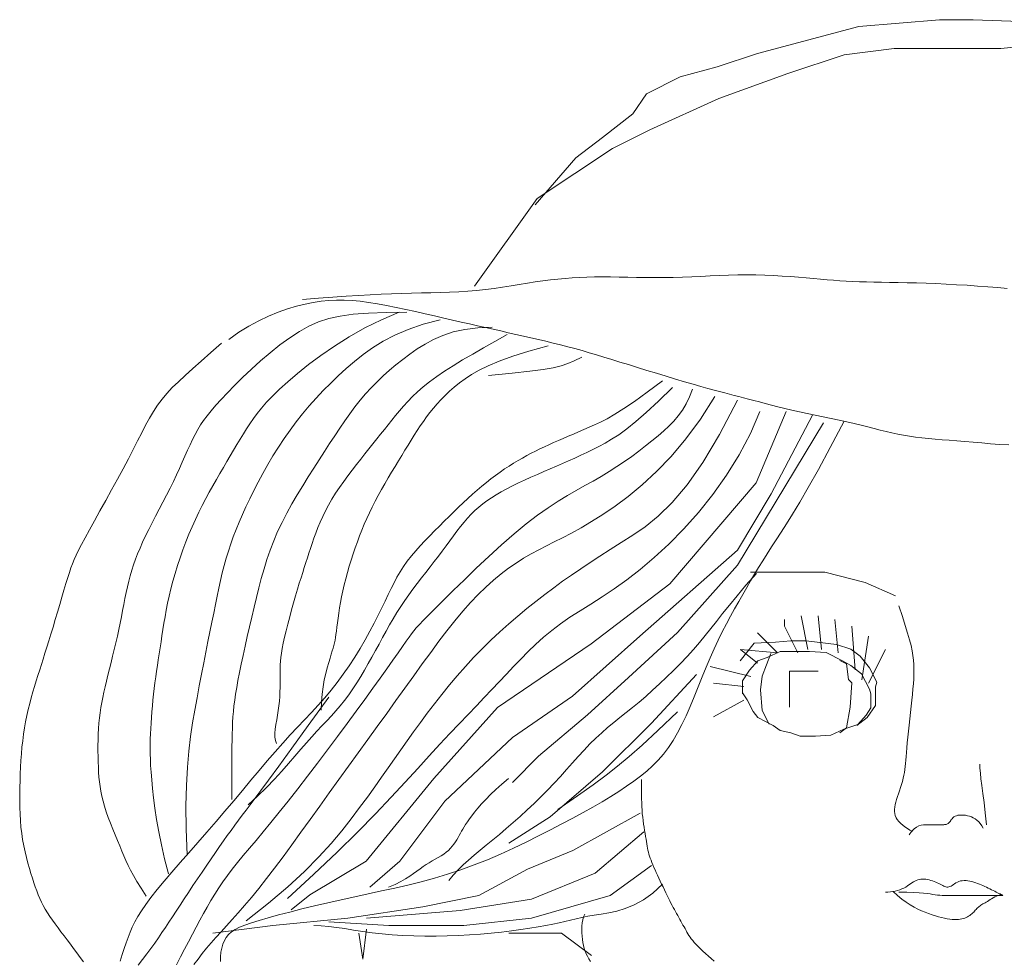
# Model space of a CAD drawing. Units: inches. Extents: x -17 to 1735, y -531 to 60.
# Tile 22 of 27: x 1734.799421 to 1734.803049, y -150.208371 to -150.204906. Entities that reach past the tile are written whole.
import ezdxf

# ---------------------------------------------------------------- set-up
doc = ezdxf.new("R2010")
doc.units = ezdxf.units.IN
doc.header["$MEASUREMENT"] = 0
doc.layers.add('A-FURN', color=242, linetype='Continuous', lineweight=18, true_color=0xcd2027)

# ---------------------------------------------------------------- blocks, each defined once
blk = doc.blocks.new('childrens_room_2')
for points in [[(73.373483, 54.431611), (73.377266, 54.43602), (73.379789, 54.437909), (73.382626, 54.440114), (73.383887, 54.442003), (73.38704, 54.443578), (73.390509, 54.444522), (73.394292, 54.445782), (73.403751, 54.448301), (73.407535, 54.448616), (73.411318, 54.448931), (73.414471, 54.448931), (73.4233, 54.448616), (73.425822, 54.448616), (73.428975, 54.447986), (73.430236, 54.447986), (73.433074, 54.446412), (73.436858, 54.445467), (73.440326, 54.443892), (73.442218, 54.441688), (73.442848, 54.442003), (73.445686, 54.439799), (73.447893, 54.437909)], [(73.367799, 54.42399), (73.373662, 54.432187), (73.380697, 54.436872), (73.384215, 54.438628), (73.390664, 54.441556), (73.397113, 54.443898), (73.402389, 54.445655), (73.407079, 54.44624), (73.41177, 54.44624), (73.417046, 54.44624), (73.422909, 54.446826), (73.428185, 54.445655), (73.429944, 54.445655), (73.436979, 54.443313), (73.440497, 54.442142), (73.446946, 54.438628), (73.449877, 54.435115), (73.453395, 54.430431), (73.453981, 54.42926)], [(73.351709, 54.422763), (73.353182, 54.422874), (73.354536, 54.422971), (73.355786, 54.423055), (73.356947, 54.423127), (73.358033, 54.423188), (73.359058, 54.423239), (73.360037, 54.423281), (73.360984, 54.423314), (73.361911, 54.423341), (73.362823, 54.423363), (73.363718, 54.423385), (73.3646, 54.423409), (73.365468, 54.42344), (73.366323, 54.42348), (73.367166, 54.423533), (73.367999, 54.423603), (73.368822, 54.423691), (73.369633, 54.423794), (73.370432, 54.423908), (73.371218, 54.424029), (73.371989, 54.424153), (73.372743, 54.424275), (73.373481, 54.42439), (73.3742, 54.424495), (73.374901, 54.424586), (73.375588, 54.424663), (73.376267, 54.424727), (73.376946, 54.424777), (73.377629, 54.424815), (73.378323, 54.424842), (73.379035, 54.424857), (73.37977, 54.424863), (73.380533, 54.424858), (73.381322, 54.424847), (73.382133, 54.424832), (73.382963, 54.424817), (73.383807, 54.424804), (73.384662, 54.424796), (73.385525, 54.424797), (73.386391, 54.42481), (73.387258, 54.424836), (73.388125, 54.424873), (73.38899, 54.424916), (73.389853, 54.424961), (73.390714, 54.425003), (73.391572, 54.425039), (73.392426, 54.425063), (73.393275, 54.425072), (73.39412, 54.425063), (73.394955, 54.425037), (73.395776, 54.424998), (73.39658, 54.424948), (73.397361, 54.424891), (73.398116, 54.424829), (73.39884, 54.424766), (73.399529, 54.424705), (73.400181, 54.424648), (73.400803, 54.424597), (73.401406, 54.42455), (73.401999, 54.424508), (73.402592, 54.424471), (73.403194, 54.424439), (73.403817, 54.424412), (73.404469, 54.42439), (73.405158, 54.424373), (73.405886, 54.424358), (73.40665, 54.424345), (73.407451, 54.424331), (73.408286, 54.424315), (73.409154, 54.424294), (73.410054, 54.424267), (73.410985, 54.424233), (73.411943, 54.424189), (73.41292, 54.424136), (73.413903, 54.424076), (73.41488, 54.42401), (73.41584, 54.423939), (73.416771, 54.423864), (73.417661, 54.423786)], [(73.34479, 54.419015), (73.345736, 54.41968), (73.346676, 54.420263), (73.347606, 54.420767), (73.348521, 54.4212), (73.349417, 54.421566), (73.350288, 54.421872), (73.35113, 54.422122), (73.351937, 54.422322), (73.352707, 54.422477), (73.353449, 54.42259), (73.354172, 54.422662), (73.354887, 54.422696), (73.355604, 54.422692), (73.356334, 54.422654), (73.357088, 54.422582), (73.357875, 54.422479), (73.358704, 54.422347), (73.359567, 54.422191), (73.360454, 54.422014), (73.361357, 54.421823), (73.362264, 54.421622), (73.363166, 54.421416), (73.364054, 54.421211), (73.364917, 54.42101), (73.365748, 54.420818), (73.366548, 54.420634), (73.367323, 54.420458), (73.368077, 54.420288), (73.368813, 54.420123), (73.369536, 54.419962), (73.37025, 54.419803), (73.37096, 54.419645), (73.371669, 54.419488), (73.372377, 54.419329), (73.373083, 54.41917), (73.373785, 54.419009), (73.374482, 54.418845), (73.375172, 54.418678), (73.375856, 54.418508), (73.37653, 54.418333), (73.377197, 54.418153), (73.377861, 54.417967), (73.378529, 54.417774), (73.37921, 54.417572), (73.379911, 54.41736), (73.380639, 54.417137), (73.381402, 54.416902), (73.382206, 54.416654), (73.383055, 54.416391), (73.383938, 54.41612), (73.384836, 54.415844), (73.385733, 54.415571), (73.386614, 54.415305), (73.38746, 54.415052), (73.388256, 54.414817), (73.388985, 54.414607), (73.389635, 54.414424), (73.390215, 54.414266), (73.390738, 54.414127), (73.391218, 54.414003), (73.391669, 54.413889), (73.392103, 54.41378), (73.392535, 54.413671), (73.392979, 54.413557), (73.393444, 54.413434), (73.393936, 54.413303), (73.394455, 54.413164), (73.395002, 54.413019), (73.395578, 54.412869), (73.396186, 54.412716), (73.396825, 54.41256), (73.397498, 54.412402), (73.398203, 54.412245), (73.398934, 54.412087), (73.399681, 54.41193), (73.400434, 54.411773), (73.401185, 54.411615), (73.401924, 54.411458), (73.402643, 54.4113), (73.403331, 54.411143), (73.403982, 54.410986), (73.4046, 54.41083), (73.405191, 54.410679), (73.405761, 54.410533), (73.406316, 54.410394), (73.406863, 54.410264), (73.407407, 54.410146), (73.407955, 54.410041), (73.408512, 54.409949), (73.409083, 54.40987), (73.409669, 54.409801), (73.410274, 54.409739), (73.410901, 54.409682), (73.411554, 54.409627), (73.412235, 54.409573), (73.412947, 54.409516), (73.413693, 54.409455), (73.41447, 54.40939), (73.415273, 54.409325), (73.4161, 54.40926), (73.416947, 54.409197), (73.41781, 54.409139)], [(73.361451, 54.421556), (73.359517, 54.421538), (73.357865, 54.421479), (73.356451, 54.421369), (73.355231, 54.421201), (73.354161, 54.420964), (73.353196, 54.420651), (73.352293, 54.420252), (73.351406, 54.419758), (73.350503, 54.419167), (73.349587, 54.418494), (73.348673, 54.417763), (73.347778, 54.416997), (73.346915, 54.416216), (73.346099, 54.415444), (73.345346, 54.414704), (73.344671, 54.414017), (73.344084, 54.413401), (73.343579, 54.412848), (73.343144, 54.412345), (73.34277, 54.411879), (73.342444, 54.411438), (73.342156, 54.411008), (73.341896, 54.410577), (73.341652, 54.410132), (73.341415, 54.409662), (73.341179, 54.409166), (73.340943, 54.408646), (73.340701, 54.408102), (73.340452, 54.407537), (73.34019, 54.406952), (73.339914, 54.406347), (73.33962, 54.405725), (73.339305, 54.405087), (73.338975, 54.404438), (73.338635, 54.403784), (73.338292, 54.40313), (73.337951, 54.402481), (73.337619, 54.401843), (73.337303, 54.401221), (73.337007, 54.400622), (73.336737, 54.400047), (73.336492, 54.399495), (73.336271, 54.398961), (73.336071, 54.39844), (73.335889, 54.397927), (73.335725, 54.397417), (73.335576, 54.396906), (73.335439, 54.396388), (73.335314, 54.395861), (73.335196, 54.395323), (73.335084, 54.394774), (73.334975, 54.394214), (73.334865, 54.393643), (73.334753, 54.393061), (73.334636, 54.392469), (73.33451, 54.391865), (73.334375, 54.391252), (73.334231, 54.390632), (73.334081, 54.390011), (73.33393, 54.389393), (73.333778, 54.388784), (73.333628, 54.388187), (73.333485, 54.387608), (73.333349, 54.387052), (73.333224, 54.386521), (73.333109, 54.386012), (73.333006, 54.385519), (73.332913, 54.385037), (73.332832, 54.38456), (73.332761, 54.384084), (73.332701, 54.383602), (73.332652, 54.383109), (73.332614, 54.382601), (73.332586, 54.382082), (73.332567, 54.381556), (73.332558, 54.381028), (73.332556, 54.380503), (73.332562, 54.379985), (73.332575, 54.37948), (73.332594, 54.378991), (73.332619, 54.378523), (73.332652, 54.37807), (73.332696, 54.377626), (73.332754, 54.377186), (73.332828, 54.376744), (73.332921, 54.376292), (73.333035, 54.375826), (73.333175, 54.375338), (73.33334, 54.374826), (73.333527, 54.374294), (73.33373, 54.37375), (73.333944, 54.373203), (73.334164, 54.37266), (73.334383, 54.372129), (73.334597, 54.371618), (73.3348, 54.371134), (73.334991, 54.370681), (73.335179, 54.370244), (73.335379, 54.369806), (73.335606, 54.369347), (73.335874, 54.368848), (73.336197, 54.368292), (73.336589, 54.367658), (73.337065, 54.366929)], [(73.360755, 54.421556), (73.359098, 54.420858), (73.35753, 54.420085), (73.356056, 54.419256), (73.354683, 54.418396), (73.353418, 54.417524), (73.352267, 54.416663), (73.351236, 54.415835), (73.350332, 54.415061), (73.349558, 54.414358), (73.3489, 54.41372), (73.348343, 54.413137), (73.347868, 54.412597), (73.347461, 54.412089), (73.347103, 54.411603), (73.346779, 54.411129), (73.346471, 54.410654), (73.346166, 54.41017), (73.345861, 54.409675), (73.345554, 54.40917), (73.345245, 54.408653), (73.344933, 54.408126), (73.344618, 54.407588), (73.344298, 54.407039), (73.343974, 54.406479), (73.343645, 54.405908), (73.343313, 54.405324), (73.342979, 54.404727), (73.342646, 54.404116), (73.342316, 54.403487), (73.34199, 54.402842), (73.341672, 54.402177), (73.341362, 54.401491), (73.341062, 54.400786), (73.340776, 54.400063), (73.340502, 54.39933), (73.340244, 54.398592), (73.340002, 54.397854), (73.339778, 54.39712), (73.339572, 54.396398), (73.339387, 54.395692), (73.339224, 54.395007), (73.339079, 54.394342), (73.338951, 54.393697), (73.338836, 54.393068), (73.338732, 54.392457), (73.338636, 54.39186), (73.338546, 54.391276), (73.338458, 54.390705), (73.338371, 54.390145), (73.338285, 54.389594), (73.3382, 54.389049), (73.338117, 54.388509), (73.338037, 54.387972), (73.33796, 54.387435), (73.337888, 54.386897), (73.33782, 54.386356), (73.337757, 54.38581), (73.3377, 54.385262), (73.337648, 54.384716), (73.337602, 54.384174), (73.337561, 54.383641), (73.337526, 54.383119), (73.337496, 54.382612), (73.337471, 54.382123), (73.337453, 54.381653), (73.337441, 54.381191), (73.337437, 54.380723), (73.337442, 54.380235), (73.337459, 54.379712), (73.337488, 54.379142), (73.33753, 54.37851), (73.337587, 54.377803), (73.337662, 54.377008), (73.337759, 54.376124), (73.337885, 54.375153), (73.338045, 54.374095), (73.338246, 54.372951), (73.338494, 54.371723), (73.338795, 54.370411), (73.339155, 54.369017)], [(73.364587, 54.42086), (73.362991, 54.420437), (73.361583, 54.419957), (73.360341, 54.419426), (73.359241, 54.418852), (73.35826, 54.418243), (73.357373, 54.417606), (73.356558, 54.416949), (73.35579, 54.416279), (73.355051, 54.415602), (73.354336, 54.414917), (73.353645, 54.414223), (73.352978, 54.413517), (73.352333, 54.412798), (73.351712, 54.412063), (73.351113, 54.41131), (73.350536, 54.410538), (73.34998, 54.409745), (73.349448, 54.408937), (73.348938, 54.408119), (73.348453, 54.407298), (73.347991, 54.406479), (73.347555, 54.405669), (73.347145, 54.404875), (73.346761, 54.404101), (73.346405, 54.403353), (73.346074, 54.402628), (73.345767, 54.401922), (73.345484, 54.401231), (73.345223, 54.40055), (73.344981, 54.399877), (73.344759, 54.399206), (73.344555, 54.398534), (73.344367, 54.397856), (73.344191, 54.397169), (73.344025, 54.396466), (73.343866, 54.395743), (73.343708, 54.394996), (73.343551, 54.39422), (73.343389, 54.39341), (73.34322, 54.392561), (73.34304, 54.39167), (73.342852, 54.390736), (73.342656, 54.389762), (73.342454, 54.388748), (73.342248, 54.387696), (73.34204, 54.386608), (73.341831, 54.385484), (73.341623, 54.384326), (73.341419, 54.38313), (73.341228, 54.381864), (73.341059, 54.380492), (73.340922, 54.378977), (73.340828, 54.377283), (73.340786, 54.375372), (73.340806, 54.373209), (73.340897, 54.370757)], [(73.369464, 54.420164), (73.368106, 54.420109), (73.366894, 54.419954), (73.365811, 54.41971), (73.364841, 54.419392), (73.363966, 54.419013), (73.363169, 54.418586), (73.362433, 54.418125), (73.361742, 54.417642), (73.36108, 54.417148), (73.360444, 54.416645), (73.359833, 54.416129), (73.359245, 54.415601), (73.358679, 54.415058), (73.358133, 54.414498), (73.357606, 54.41392), (73.357097, 54.413321), (73.356603, 54.412702), (73.356122, 54.41206), (73.355649, 54.411397), (73.355181, 54.410712), (73.354712, 54.410005), (73.354239, 54.409277), (73.353758, 54.408526), (73.353265, 54.407754), (73.352757, 54.406961), (73.35224, 54.406149), (73.351722, 54.40532), (73.351211, 54.404478), (73.350712, 54.403625), (73.350235, 54.402764), (73.349787, 54.401897), (73.349374, 54.401028), (73.349003, 54.400157), (73.34867, 54.399286), (73.34837, 54.398412), (73.348097, 54.397534), (73.347846, 54.39665), (73.347611, 54.39576), (73.347387, 54.394861), (73.347168, 54.393953), (73.346951, 54.393036), (73.346736, 54.392117), (73.346527, 54.391207), (73.346326, 54.390314), (73.346136, 54.389448), (73.345959, 54.38862), (73.345799, 54.387837), (73.345658, 54.38711), (73.345538, 54.386445), (73.345438, 54.385833), (73.345355, 54.385264), (73.345288, 54.384725), (73.345235, 54.384205), (73.345193, 54.383693), (73.345161, 54.383177), (73.345136, 54.382645), (73.345117, 54.382089), (73.345102, 54.381514), (73.345092, 54.38093), (73.345085, 54.380343), (73.345081, 54.379764), (73.345079, 54.379199), (73.345078, 54.378659), (73.345078, 54.378151), (73.345078, 54.377682), (73.345078, 54.37726), (73.345078, 54.376889), (73.345078, 54.376574), (73.345078, 54.37632), (73.345078, 54.376132), (73.345078, 54.376016), (73.345078, 54.375976)], [(73.344126, 54.418666), (73.34312, 54.417778), (73.342222, 54.41699), (73.341422, 54.416286), (73.340711, 54.415648), (73.340079, 54.41506), (73.339515, 54.414504), (73.339011, 54.413962), (73.338556, 54.413418), (73.338141, 54.412856), (73.337753, 54.412268), (73.337383, 54.411648), (73.337019, 54.41099), (73.33665, 54.410288), (73.336265, 54.409536), (73.335853, 54.408727), (73.335403, 54.407855), (73.334908, 54.406919), (73.334379, 54.405938), (73.333832, 54.404937), (73.333282, 54.403938), (73.332743, 54.402967), (73.332233, 54.402046), (73.331766, 54.401201), (73.331357, 54.400454), (73.331017, 54.399823), (73.33074, 54.399289), (73.330514, 54.398828), (73.330326, 54.398414), (73.330165, 54.398022), (73.330019, 54.397628), (73.329878, 54.397205), (73.329728, 54.396728), (73.329561, 54.39618), (73.329378, 54.395568), (73.329183, 54.394908), (73.328979, 54.394215), (73.32877, 54.393506), (73.32856, 54.392794), (73.328353, 54.392096), (73.328151, 54.391427), (73.327959, 54.390799), (73.327775, 54.390208), (73.327599, 54.389648), (73.327429, 54.389111), (73.327264, 54.388592), (73.327102, 54.388084), (73.326943, 54.387579), (73.326785, 54.387071), (73.326628, 54.386554), (73.326472, 54.386028), (73.32632, 54.385492), (73.326174, 54.384945), (73.326035, 54.384389), (73.325906, 54.383824), (73.325787, 54.383248), (73.325682, 54.382662), (73.32559, 54.382067), (73.325512, 54.381464), (73.325447, 54.380852), (73.325393, 54.380235), (73.325348, 54.379613), (73.325312, 54.378987), (73.325284, 54.378359), (73.325261, 54.377729), (73.325244, 54.377099), (73.325234, 54.376471), (73.325233, 54.375845), (73.325241, 54.375223), (73.325263, 54.374606), (73.325298, 54.373994), (73.32535, 54.373391), (73.325419, 54.372796), (73.325507, 54.37221), (73.325612, 54.371638), (73.32573, 54.37108), (73.325859, 54.370539), (73.325995, 54.370018), (73.326136, 54.369519), (73.326277, 54.369044), (73.326417, 54.368597), (73.326553, 54.368178), (73.326687, 54.367784), (73.326823, 54.367411), (73.326962, 54.367055), (73.32711, 54.366711), (73.327267, 54.366375), (73.327438, 54.366043), (73.327626, 54.36571), (73.327832, 54.365373), (73.328057, 54.36503), (73.328297, 54.364682), (73.328552, 54.364326), (73.328819, 54.363963), (73.329096, 54.363592), (73.329383, 54.363212), (73.329675, 54.362824), (73.329973, 54.362426), (73.330275, 54.36202), (73.33058, 54.36161), (73.330887, 54.361197), (73.331196, 54.360784)], [(73.370858, 54.419468), (73.369715, 54.418832), (73.368638, 54.418225), (73.367627, 54.417646), (73.366684, 54.417091), (73.365809, 54.416558), (73.365003, 54.416043), (73.364266, 54.415545), (73.3636, 54.415061), (73.363002, 54.414588), (73.362467, 54.414124), (73.361984, 54.413669), (73.361546, 54.41322), (73.361143, 54.412777), (73.360766, 54.412337), (73.360408, 54.411901), (73.360058, 54.411466), (73.359709, 54.41103), (73.359359, 54.410593), (73.359007, 54.410152), (73.35865, 54.409704), (73.358288, 54.409249), (73.357919, 54.408783), (73.357541, 54.408305), (73.357155, 54.407812), (73.356758, 54.407305), (73.356356, 54.406783), (73.355954, 54.406251), (73.355558, 54.40571), (73.355172, 54.405164), (73.354803, 54.404616), (73.354456, 54.404067), (73.354135, 54.403521), (73.353846, 54.40298), (73.353587, 54.402447), (73.353353, 54.401921), (73.353141, 54.401405), (73.352949, 54.400899), (73.352772, 54.400406), (73.352607, 54.399926), (73.352452, 54.399462), (73.352302, 54.399012), (73.352155, 54.39857), (73.35201, 54.398129), (73.351864, 54.397679), (73.351715, 54.397212), (73.351562, 54.396722), (73.351401, 54.396199), (73.351232, 54.395635), (73.351053, 54.395025), (73.350869, 54.394381), (73.350682, 54.393717), (73.350499, 54.393047), (73.350324, 54.392384), (73.350163, 54.391745), (73.350019, 54.391142), (73.349897, 54.390589), (73.349801, 54.390098), (73.349729, 54.389662), (73.349677, 54.389268), (73.349643, 54.388908), (73.349622, 54.388569), (73.349611, 54.388241), (73.349607, 54.387913), (73.349607, 54.387574), (73.349606, 54.387215), (73.349604, 54.386838), (73.349597, 54.386443), (73.349585, 54.386034), (73.349564, 54.385612), (73.349533, 54.38518), (73.34949, 54.384742), (73.349432, 54.384297), (73.349361, 54.383851), (73.349283, 54.383409), (73.349209, 54.382977), (73.349149, 54.382561), (73.349114, 54.382169), (73.349114, 54.381806), (73.349158, 54.381479), (73.349258, 54.381195)], [(73.37469, 54.418425), (73.372887, 54.417918), (73.371376, 54.417441), (73.370118, 54.416987), (73.369079, 54.416554), (73.368223, 54.416138), (73.367513, 54.415733), (73.366913, 54.415337), (73.366387, 54.414945), (73.365904, 54.414554), (73.365457, 54.414161), (73.365041, 54.413768), (73.364652, 54.413372), (73.364288, 54.412974), (73.363945, 54.412572), (73.36362, 54.412166), (73.363309, 54.411756), (73.36301, 54.41134), (73.362718, 54.410917), (73.362432, 54.410486), (73.362148, 54.410045), (73.361865, 54.409594), (73.361578, 54.40913), (73.361287, 54.408653), (73.360987, 54.40816), (73.360677, 54.407652), (73.36036, 54.407131), (73.360039, 54.406599), (73.359717, 54.406058), (73.359398, 54.405512), (73.359084, 54.404964), (73.358781, 54.404415), (73.35849, 54.403869), (73.358215, 54.403328), (73.357955, 54.40279), (73.357708, 54.402253), (73.357474, 54.401716), (73.357251, 54.401176), (73.357037, 54.400632), (73.356831, 54.40008), (73.356632, 54.39952), (73.356439, 54.39895), (73.356253, 54.398372), (73.356075, 54.39779), (73.355906, 54.397207), (73.355749, 54.396628), (73.355603, 54.396054), (73.355472, 54.39549), (73.355355, 54.394939), (73.355254, 54.394404), (73.355167, 54.393888), (73.355092, 54.393396), (73.355028, 54.392931), (73.354972, 54.392495), (73.354922, 54.392093), (73.354876, 54.391727), (73.354832, 54.391401), (73.354788, 54.391116), (73.354742, 54.390861), (73.354691, 54.390622), (73.354633, 54.390386), (73.354565, 54.39014), (73.354485, 54.389868), (73.354391, 54.389559), (73.354281, 54.389198), (73.354153, 54.388774), (73.354014, 54.38829), (73.353874, 54.387748), (73.35374, 54.387153), (73.353621, 54.38651), (73.353525, 54.385822), (73.353462, 54.385092), (73.353439, 54.384326)], [(73.377831, 54.417364), (73.377128, 54.417018), (73.376519, 54.416749), (73.375902, 54.416538), (73.375174, 54.416363), (73.374235, 54.416205), (73.372981, 54.416043), (73.37131, 54.415856), (73.369121, 54.415624)], [(73.385382, 54.415149), (73.383965, 54.414081), (73.382769, 54.413221), (73.381764, 54.412539), (73.380918, 54.412006), (73.380202, 54.411594), (73.379584, 54.411274), (73.379035, 54.411016), (73.378524, 54.410792), (73.378025, 54.410578), (73.377534, 54.410368), (73.377051, 54.410162), (73.376576, 54.409959), (73.37611, 54.409759), (73.375653, 54.40956), (73.375205, 54.409362), (73.374767, 54.409165), (73.374338, 54.408968), (73.373917, 54.408769), (73.373502, 54.408567), (73.373092, 54.408359), (73.372684, 54.408143), (73.372276, 54.407918), (73.371868, 54.407682), (73.371456, 54.407433), (73.37104, 54.40717), (73.370619, 54.406892), (73.370195, 54.406599), (73.369768, 54.406292), (73.369338, 54.40597), (73.368907, 54.405633), (73.368474, 54.405281), (73.36804, 54.404914), (73.367607, 54.404533), (73.367172, 54.404139), (73.366737, 54.403732), (73.3663, 54.403314), (73.36586, 54.402886), (73.365417, 54.402449), (73.36497, 54.402005), (73.36452, 54.401555), (73.364065, 54.4011), (73.36361, 54.40064), (73.36316, 54.400175), (73.36272, 54.399705), (73.362294, 54.39923), (73.361889, 54.398751), (73.361508, 54.398266), (73.361156, 54.397777), (73.360837, 54.397281), (73.360543, 54.396775), (73.360265, 54.396253), (73.359994, 54.39571), (73.35972, 54.39514), (73.359435, 54.394536), (73.359128, 54.393895), (73.358792, 54.39321), (73.358418, 54.392479), (73.358007, 54.39171), (73.357564, 54.390913), (73.35709, 54.390101), (73.35659, 54.389283), (73.356065, 54.388472), (73.355519, 54.387678), (73.354955, 54.386912), (73.354377, 54.386182), (73.353782, 54.385481), (73.353172, 54.384796), (73.352545, 54.384118), (73.351901, 54.383434), (73.351238, 54.382735), (73.350558, 54.382009), (73.349858, 54.381244), (73.349139, 54.380433), (73.348401, 54.379579), (73.347644, 54.378689), (73.346869, 54.377767), (73.346078, 54.376821), (73.345269, 54.375856), (73.344445, 54.37488), (73.343605, 54.373896), (73.342752, 54.372914), (73.341899, 54.371941), (73.341057, 54.370986), (73.340242, 54.370059), (73.339465, 54.369168), (73.338742, 54.368324), (73.338086, 54.367535), (73.337509, 54.366811), (73.337022, 54.366157), (73.336616, 54.365564), (73.336279, 54.365019), (73.335998, 54.364508), (73.335762, 54.36402), (73.335558, 54.363542), (73.335374, 54.363059), (73.335197, 54.36256), (73.335016, 54.362032), (73.334826, 54.361463), (73.33462, 54.360842)], [(73.38819, 54.414374), (73.38791, 54.413632), (73.387596, 54.412974), (73.387249, 54.412387), (73.386866, 54.411854), (73.386448, 54.411363), (73.385993, 54.410899), (73.385502, 54.410447), (73.384973, 54.409992), (73.384406, 54.409525), (73.383804, 54.409046), (73.38317, 54.40856), (73.382509, 54.408072), (73.381823, 54.407587), (73.381115, 54.407109), (73.38039, 54.406644), (73.37965, 54.406195), (73.378897, 54.405765), (73.378126, 54.405337), (73.377326, 54.404893), (73.376492, 54.404414), (73.375613, 54.403879), (73.374682, 54.403271), (73.373691, 54.402569), (73.372631, 54.401756), (73.371501, 54.40082), (73.370326, 54.399791), (73.369138, 54.398708), (73.367967, 54.397608), (73.366845, 54.39653), (73.365804, 54.395512), (73.364876, 54.394593), (73.364092, 54.393811), (73.363472, 54.393192), (73.362997, 54.392712), (73.362634, 54.392336), (73.362352, 54.392029), (73.362119, 54.391755), (73.361904, 54.391478), (73.361675, 54.391163), (73.361401, 54.390773), (73.361056, 54.390281), (73.360637, 54.389685), (73.360147, 54.388991), (73.359588, 54.388203), (73.358963, 54.387328), (73.358276, 54.38637), (73.357528, 54.385336), (73.356722, 54.384231), (73.355864, 54.383062), (73.354965, 54.381848), (73.35404, 54.38061), (73.353103, 54.379368), (73.352169, 54.378142), (73.351252, 54.376952), (73.350367, 54.375821), (73.349528, 54.374767), (73.348746, 54.373807), (73.348021, 54.372934), (73.347349, 54.372135), (73.346728, 54.371401), (73.346153, 54.370719), (73.345621, 54.370077), (73.345129, 54.369463), (73.344673, 54.368867), (73.34425, 54.368278), (73.343854, 54.367691), (73.34348, 54.367102), (73.343123, 54.366509), (73.342777, 54.365907), (73.342436, 54.365294), (73.342095, 54.364665), (73.341749, 54.364019), (73.341393, 54.363351), (73.341028, 54.362663), (73.340656, 54.361958), (73.340279, 54.361237), (73.3399, 54.360502)], [(73.386328, 54.414519), (73.385008, 54.413229), (73.38387, 54.412174), (73.382889, 54.411322), (73.382038, 54.410642), (73.381294, 54.410101), (73.38063, 54.40967), (73.380022, 54.409316), (73.379444, 54.409008), (73.378874, 54.40872), (73.378308, 54.408444), (73.377743, 54.408178), (73.377177, 54.407919), (73.376609, 54.407665), (73.376037, 54.407414), (73.375458, 54.407162), (73.374872, 54.406909), (73.374277, 54.40665), (73.373677, 54.406388), (73.373079, 54.406122), (73.372487, 54.405852), (73.371908, 54.405581), (73.371347, 54.405307), (73.370809, 54.405032), (73.3703, 54.404757), (73.369824, 54.404481), (73.369379, 54.404202), (73.368961, 54.403916), (73.368566, 54.403622), (73.368191, 54.403315), (73.367832, 54.402993), (73.367485, 54.402652), (73.367147, 54.40229), (73.366814, 54.401904), (73.366484, 54.401496), (73.366153, 54.401069), (73.36582, 54.400624), (73.365482, 54.400164), (73.365137, 54.399692), (73.364782, 54.39921), (73.364414, 54.398721), (73.364033, 54.398227), (73.363641, 54.397726), (73.363241, 54.39722), (73.362838, 54.396707), (73.362435, 54.396187), (73.362035, 54.395658), (73.361643, 54.395121), (73.361261, 54.394575), (73.360894, 54.394019), (73.360539, 54.393454), (73.360194, 54.39288), (73.359856, 54.392299), (73.359523, 54.391709), (73.359192, 54.391114), (73.358862, 54.390512), (73.358529, 54.389904), (73.358191, 54.389292), (73.357848, 54.38868), (73.357499, 54.388071), (73.357143, 54.38747), (73.356779, 54.386882), (73.356408, 54.38631), (73.356028, 54.385759), (73.355639, 54.385233), (73.355239, 54.384734), (73.354829, 54.384256), (73.354406, 54.383788), (73.35397, 54.383321), (73.353519, 54.382845), (73.353052, 54.382351), (73.352568, 54.381829), (73.352065, 54.38127), (73.351542, 54.380667), (73.35099, 54.380021), (73.350401, 54.379336), (73.349766, 54.378617), (73.349078, 54.377866), (73.348326, 54.377089), (73.347503, 54.37629), (73.3466, 54.375471)], [(73.390295, 54.413673), (73.388958, 54.411567), (73.38759, 54.409705), (73.38621, 54.408069), (73.384837, 54.406641), (73.383491, 54.405401), (73.382189, 54.404332), (73.380952, 54.403415), (73.379796, 54.402632), (73.378737, 54.401963), (73.377767, 54.401391), (73.376873, 54.400898), (73.376042, 54.400463), (73.375262, 54.40007), (73.37452, 54.399699), (73.373803, 54.399333), (73.373099, 54.398952), (73.372397, 54.39854), (73.371695, 54.398092), (73.37099, 54.397602), (73.370284, 54.397068), (73.369576, 54.396484), (73.368863, 54.395846), (73.368147, 54.395152), (73.367426, 54.394395), (73.366699, 54.393575), (73.365964, 54.392693), (73.36522, 54.391755), (73.364465, 54.390766), (73.363695, 54.38973), (73.36291, 54.388653), (73.362107, 54.387539), (73.361284, 54.386392), (73.36044, 54.385218), (73.359578, 54.384021), (73.358701, 54.382804), (73.357811, 54.381573), (73.356914, 54.38033), (73.356012, 54.379081), (73.355108, 54.377829), (73.354207, 54.376578), (73.353311, 54.375334), (73.352426, 54.374106), (73.351555, 54.372903), (73.350705, 54.371737), (73.349879, 54.370617), (73.349083, 54.369555), (73.348321, 54.368559), (73.347598, 54.36764), (73.346917, 54.366806), (73.346278, 54.36605), (73.345677, 54.36536), (73.345112, 54.364727), (73.344579, 54.364141), (73.344077, 54.363591), (73.343602, 54.363067), (73.343152, 54.362558), (73.342724, 54.362056), (73.342315, 54.361552), (73.341923, 54.361041), (73.341544, 54.360514)], [(73.392401, 54.413322), (73.390739, 54.410105), (73.389171, 54.407495), (73.387694, 54.405411), (73.386303, 54.403771), (73.384995, 54.402492), (73.383764, 54.401493), (73.382608, 54.40069), (73.381522, 54.400003), (73.3805, 54.399361), (73.379535, 54.398744), (73.378616, 54.398146), (73.377735, 54.397557), (73.37688, 54.396971), (73.376044, 54.39638), (73.375216, 54.395777), (73.374386, 54.395155), (73.373548, 54.394506), (73.372703, 54.39383), (73.371855, 54.393129), (73.371008, 54.392402), (73.370167, 54.39165), (73.369336, 54.390875), (73.368518, 54.390076), (73.367718, 54.389255), (73.366939, 54.388412), (73.366183, 54.387552), (73.365448, 54.38668), (73.364735, 54.385801), (73.364044, 54.384918), (73.363375, 54.384038), (73.362728, 54.383165), (73.362103, 54.382303), (73.361498, 54.381455), (73.360905, 54.380615), (73.360315, 54.379772), (73.359716, 54.378919), (73.359099, 54.378044), (73.358455, 54.37714), (73.357773, 54.376197), (73.357044, 54.375205), (73.356253, 54.374157), (73.355373, 54.373044), (73.354371, 54.371858), (73.353216, 54.370594), (73.351876, 54.369244), (73.35032, 54.3678), (73.348514, 54.366255), (73.346428, 54.364603)], [(73.394507, 54.412271), (73.393624, 54.410203), (73.392575, 54.408212), (73.391394, 54.406313), (73.390112, 54.404516), (73.388762, 54.402834), (73.387375, 54.401279), (73.385984, 54.399864), (73.384622, 54.398601), (73.383314, 54.397496), (73.382066, 54.396533), (73.380879, 54.395687), (73.379752, 54.394936), (73.378686, 54.394255), (73.37768, 54.393623), (73.376734, 54.393015), (73.375848, 54.392409), (73.375021, 54.391785), (73.374245, 54.391141), (73.37351, 54.39048), (73.372807, 54.389802), (73.372125, 54.389111), (73.371456, 54.388408), (73.37079, 54.387696), (73.370116, 54.386976), (73.369427, 54.386249), (73.368714, 54.385504), (73.367972, 54.384732), (73.367192, 54.38392), (73.366368, 54.383058), (73.365494, 54.382134), (73.364562, 54.381136), (73.363565, 54.380054), (73.362493, 54.378875), (73.361318, 54.377586), (73.360007, 54.376172), (73.358528, 54.374618), (73.356849, 54.372909), (73.354937, 54.37103), (73.352761, 54.368967), (73.350288, 54.366706)], [(73.396963, 54.412271), (73.394156, 54.405611), (73.386084, 54.396148), (73.378714, 54.39054), (73.369941, 54.384581), (73.363975, 54.377922), (73.357658, 54.370211), (73.352394, 54.367056), (73.350639, 54.365654)], [(73.402408, 54.41137), (73.401096, 54.408888), (73.39998, 54.406834), (73.399037, 54.405152), (73.39824, 54.403783), (73.397565, 54.402668), (73.396987, 54.401749), (73.396482, 54.400969), (73.396023, 54.400269), (73.39559, 54.399601), (73.395176, 54.39895), (73.394777, 54.398311), (73.394391, 54.397681), (73.394013, 54.397055), (73.39364, 54.396428), (73.393269, 54.395795), (73.392896, 54.395152), (73.39252, 54.394495), (73.392139, 54.39382), (73.391756, 54.393124), (73.391372, 54.392404), (73.390988, 54.391656), (73.390606, 54.390879), (73.390225, 54.390068), (73.389848, 54.389222), (73.389476, 54.388338), (73.389106, 54.387429), (73.388736, 54.386508), (73.388364, 54.385587), (73.387987, 54.384682), (73.387602, 54.383804), (73.387207, 54.382969), (73.386801, 54.382189), (73.386379, 54.381474), (73.385938, 54.380819), (73.385476, 54.380216), (73.384988, 54.379657), (73.38447, 54.379131), (73.383919, 54.378631), (73.38333, 54.378149), (73.382702, 54.377675), (73.382029, 54.377203), (73.381311, 54.376727), (73.380546, 54.376247), (73.379733, 54.37576), (73.37887, 54.375262), (73.377957, 54.374753), (73.376993, 54.374228), (73.375975, 54.373687), (73.374905, 54.373127), (73.373788, 54.372557), (73.372631, 54.371983), (73.371443, 54.371417), (73.37023, 54.370865), (73.368999, 54.370336), (73.367759, 54.369839), (73.366516, 54.369383), (73.365277, 54.368973), (73.364041, 54.368605), (73.362806, 54.368272), (73.36157, 54.367966), (73.360332, 54.367679), (73.35909, 54.367405), (73.357841, 54.367136), (73.356585, 54.366864), (73.355321, 54.366584), (73.354065, 54.366298), (73.352834, 54.366009), (73.351645, 54.365722), (73.350515, 54.36544), (73.349461, 54.365166), (73.3485, 54.364905), (73.347651, 54.364659), (73.346925, 54.364432), (73.346314, 54.364217), (73.345807, 54.364006), (73.345391, 54.363793), (73.345054, 54.363571), (73.344784, 54.363331), (73.344567, 54.363066), (73.344393, 54.36277), (73.344251, 54.362436), (73.34414, 54.362067), (73.344064, 54.361667), (73.344025, 54.361241), (73.344026, 54.360793)], [(73.39942, 54.41192), (73.395559, 54.40456), (73.392401, 54.399302), (73.383276, 54.391241), (73.37696, 54.385633), (73.371345, 54.381777), (73.365028, 54.375819), (73.360816, 54.370211), (73.358009, 54.367757)], [(73.400472, 54.411219), (73.392401, 54.3979), (73.386786, 54.391591), (73.382224, 54.387385), (73.378363, 54.38388), (73.373801, 54.380025), (73.371345, 54.377571)], [(73.39418, 54.397123), (73.393205, 54.396011), (73.392369, 54.395026), (73.391647, 54.394149), (73.391014, 54.393359), (73.390444, 54.392636), (73.389911, 54.39196), (73.389391, 54.391311), (73.388857, 54.390668), (73.388291, 54.390016), (73.387693, 54.389357), (73.38707, 54.388697), (73.38643, 54.388043), (73.385778, 54.387401), (73.385123, 54.386778), (73.38447, 54.386181), (73.383827, 54.385615), (73.383199, 54.385085), (73.382586, 54.384585), (73.381987, 54.384105), (73.3814, 54.383636), (73.380824, 54.383171), (73.380257, 54.382699), (73.379699, 54.382212), (73.379148, 54.381701), (73.378602, 54.38116), (73.378058, 54.38059), (73.377512, 54.379998), (73.376962, 54.379386), (73.376403, 54.378762), (73.375833, 54.378128), (73.375248, 54.37749), (73.374644, 54.376853), (73.37402, 54.376221), (73.373379, 54.375597), (73.372728, 54.374984), (73.372071, 54.374385), (73.371413, 54.373802), (73.370762, 54.373238), (73.370121, 54.372696), (73.369497, 54.372179), (73.368894, 54.371688), (73.368314, 54.371216), (73.367759, 54.370757), (73.36723, 54.370303), (73.366729, 54.369846), (73.366256, 54.369378), (73.365814, 54.368893), (73.365403, 54.368382)], [(73.4072, 54.395023), (73.404362, 54.396283), (73.400579, 54.397228), (73.398056, 54.397228), (73.394588, 54.397228), (73.393642, 54.397228)], [(73.407515, 54.394079), (73.407841, 54.393094), (73.408113, 54.39225), (73.408335, 54.391528), (73.408514, 54.390907), (73.408652, 54.390365), (73.408757, 54.389883), (73.408831, 54.389439), (73.408881, 54.389014), (73.408911, 54.388589), (73.408923, 54.388158), (73.408919, 54.387718), (73.408901, 54.387266), (73.408871, 54.386797), (73.40883, 54.386309), (73.40878, 54.385798), (73.408724, 54.385261), (73.408663, 54.384697), (73.408598, 54.384114), (73.408533, 54.383522), (73.408468, 54.382932), (73.408405, 54.382355), (73.408347, 54.3818), (73.408295, 54.381278), (73.408251, 54.3808), (73.408216, 54.380373), (73.408188, 54.379993), (73.408163, 54.37965), (73.408139, 54.379337), (73.408113, 54.379047), (73.408081, 54.378771), (73.40804, 54.378501), (73.407988, 54.378229), (73.407922, 54.377949), (73.407844, 54.377662), (73.407758, 54.377372), (73.407666, 54.377081), (73.407572, 54.376792), (73.407478, 54.376509), (73.407388, 54.376235), (73.407305, 54.375972), (73.407232, 54.375723), (73.407171, 54.375488), (73.407127, 54.375264), (73.407101, 54.37505), (73.407098, 54.374845), (73.40712, 54.374647), (73.407171, 54.374455), (73.407252, 54.374266), (73.407367, 54.374081), (73.407513, 54.373899), (73.407684, 54.373723), (73.407876, 54.373554), (73.408086, 54.373394), (73.408309, 54.373244), (73.408541, 54.373105), (73.408776, 54.37298)], [(73.398061, 54.389675), (73.3968, 54.392194), (73.3968, 54.392824)], [(73.399007, 54.38999), (73.398376, 54.393139)], [(73.400268, 54.38999), (73.399953, 54.393139)], [(73.401844, 54.389675), (73.401529, 54.392824)], [(73.403421, 54.3881), (73.403106, 54.392194)], [(73.392701, 54.38999), (73.396169, 54.389675), (73.394277, 54.391564)], [(73.404051, 54.387156), (73.404682, 54.391249)], [(73.392648, 54.388934), (73.393971, 54.390587), (73.395956, 54.390697), (73.39739, 54.390807), (73.398824, 54.390807), (73.401691, 54.390477), (73.403015, 54.390036), (73.403897, 54.389375), (73.404779, 54.388274), (73.405441, 54.386952), (73.405331, 54.386511), (73.405331, 54.384749), (73.404559, 54.383647), (73.403566, 54.382876)], [(73.394277, 54.38873), (73.392701, 54.38999)], [(73.392868, 54.38585), (73.392868, 54.387062), (73.39353, 54.388053), (73.394302, 54.388934), (73.395184, 54.389265), (73.396397, 54.389816), (73.397721, 54.389816), (73.399155, 54.389816), (73.400699, 54.389706), (73.402243, 54.388934), (73.403015, 54.388494), (73.404007, 54.387723), (73.404779, 54.386291), (73.40489, 54.38585), (73.40489, 54.384529), (73.404448, 54.383868), (73.403676, 54.382986), (73.402353, 54.382546), (73.40114, 54.381995), (73.399706, 54.381885), (73.398272, 54.381885), (73.39739, 54.382215), (73.396397, 54.382436), (73.395736, 54.382876), (73.394302, 54.383647), (73.393861, 54.384198), (73.393309, 54.3853), (73.392868, 54.38596)], [(73.395526, 54.389614), (73.394719, 54.387518), (73.394558, 54.386229), (73.394719, 54.384295), (73.395365, 54.383005)], [(73.404682, 54.386841), (73.406259, 54.38999)], [(73.393647, 54.387471), (73.389863, 54.388415)], [(73.401981, 54.388969), (73.402627, 54.388647), (73.402788, 54.387196), (73.403111, 54.386874), (73.40295, 54.384617), (73.402627, 54.382683), (73.401981, 54.382199)], [(73.388565, 54.38766), (73.384353, 54.383103), (73.379791, 54.378547), (73.374878, 54.374341), (73.371018, 54.371887)], [(73.399959, 54.387965), (73.397264, 54.387965), (73.397264, 54.384601), (73.397264, 54.384601)], [(73.393016, 54.386526), (73.390178, 54.386841)], [(73.354167, 54.385548), (73.352245, 54.382886), (73.350699, 54.380755), (73.349477, 54.379081), (73.348528, 54.37779), (73.347799, 54.376808), (73.347239, 54.37606), (73.346796, 54.375473), (73.346416, 54.374972), (73.346057, 54.374495), (73.345706, 54.374025), (73.34536, 54.373555), (73.345014, 54.37308), (73.344664, 54.372593), (73.344306, 54.37209), (73.343937, 54.371564), (73.343552, 54.37101), (73.343149, 54.370423), (73.342732, 54.369811), (73.342306, 54.369181), (73.341877, 54.368543), (73.341451, 54.367905), (73.341032, 54.367275), (73.340627, 54.366663), (73.340242, 54.366076), (73.339878, 54.365522), (73.339534, 54.364995), (73.339201, 54.364489), (73.338875, 54.363997), (73.338549, 54.363512), (73.338217, 54.363028), (73.337872, 54.362538), (73.337509, 54.362035), (73.337124, 54.361515), (73.336728, 54.360986), (73.336333, 54.360459)], [(73.393016, 54.385266), (73.390178, 54.383692)], [(73.38681, 54.384155), (73.384946, 54.382412), (73.383476, 54.381055), (73.38227, 54.379977), (73.381195, 54.379072), (73.38012, 54.378233), (73.378914, 54.377353), (73.377444, 54.376325), (73.37558, 54.375042)], [(73.415713, 54.37361), (73.415595, 54.374719), (73.415481, 54.375691), (73.415375, 54.376538), (73.415279, 54.377271), (73.415199, 54.3779), (73.415137, 54.378437), (73.415096, 54.378893), (73.415082, 54.379278)], [(73.370994, 54.377922), (73.370368, 54.377405), (73.369805, 54.376906), (73.3693, 54.376429), (73.368851, 54.375976), (73.368455, 54.375548), (73.368107, 54.375149), (73.367804, 54.374781), (73.367543, 54.374446), (73.36732, 54.374145), (73.36713, 54.373875), (73.366967, 54.37363), (73.366826, 54.373405), (73.366702, 54.373196), (73.366589, 54.372996), (73.366481, 54.372801), (73.366373, 54.372606), (73.36626, 54.372406), (73.36614, 54.372203), (73.36601, 54.371999), (73.365868, 54.371795), (73.365713, 54.371594), (73.365542, 54.371398), (73.365353, 54.371209), (73.365145, 54.371029), (73.364915, 54.370858), (73.364667, 54.370695), (73.364403, 54.370537), (73.364128, 54.370379), (73.363845, 54.370218), (73.363557, 54.370051), (73.363268, 54.369875), (73.36298, 54.369685), (73.362696, 54.36948), (73.362404, 54.369261), (73.362091, 54.369029), (73.361745, 54.368787), (73.361352, 54.368537), (73.360899, 54.36828), (73.360374, 54.36802), (73.359763, 54.367757)], [(73.383422, 54.377848), (73.383423, 54.377329), (73.383424, 54.376857), (73.383427, 54.376425), (73.383433, 54.376026), (73.383442, 54.375654), (73.383456, 54.375303), (73.383477, 54.374967), (73.383503, 54.374637), (73.383537, 54.374311), (73.383577, 54.373988), (73.383621, 54.373672), (73.383668, 54.373363), (73.383716, 54.373065), (73.383764, 54.372781), (73.38381, 54.372512), (73.383853, 54.37226), (73.383891, 54.372028), (73.383926, 54.371812), (73.38396, 54.37161), (73.383994, 54.371417), (73.384031, 54.371231), (73.384072, 54.371047), (73.38412, 54.370863), (73.384176, 54.370675), (73.384241, 54.37048), (73.384316, 54.370277), (73.3844, 54.370066), (73.384492, 54.369846), (73.384591, 54.369617), (73.384698, 54.369379), (73.38481, 54.369132), (73.384929, 54.368875), (73.385052, 54.368609), (73.385179, 54.368336), (73.385309, 54.368058), (73.38544, 54.367781), (73.385571, 54.367505), (73.3857, 54.367236), (73.385827, 54.366975), (73.385951, 54.366726), (73.386069, 54.366492), (73.386184, 54.36627), (73.386294, 54.366061), (73.386401, 54.36586), (73.386506, 54.365667), (73.386609, 54.36548), (73.38671, 54.365296), (73.386811, 54.365115), (73.386912, 54.364933), (73.387013, 54.364753), (73.387113, 54.364573), (73.387212, 54.364396), (73.387309, 54.364221), (73.387405, 54.364049), (73.387499, 54.363881), (73.387591, 54.363718), (73.387682, 54.363559), (73.387773, 54.363402), (73.387868, 54.363247), (73.387971, 54.36309), (73.388086, 54.362929), (73.388216, 54.362762), (73.388363, 54.362587), (73.388533, 54.362401), (73.388726, 54.362204), (73.388942, 54.361995), (73.389175, 54.361778), (73.389424, 54.361552), (73.389684, 54.36132), (73.389951, 54.361083), (73.390223, 54.360843)], [(73.383301, 54.374691), (73.376984, 54.371186), (73.372772, 54.369434), (73.36821, 54.36698), (73.362946, 54.365929), (73.355927, 54.364877), (73.348909, 54.364176), (73.343293, 54.363475)], [(73.408461, 54.372665), (73.408697, 54.372977), (73.408932, 54.373212), (73.409162, 54.373379), (73.409387, 54.373492), (73.409605, 54.37356), (73.409813, 54.373595), (73.410011, 54.373608), (73.410195, 54.37361), (73.410365, 54.37361), (73.410521, 54.37361), (73.410664, 54.37361), (73.410793, 54.37361), (73.41091, 54.37361), (73.411015, 54.37361), (73.41111, 54.37361), (73.411194, 54.37361), (73.411268, 54.37361), (73.411334, 54.37361), (73.411394, 54.37361), (73.41145, 54.37361), (73.411503, 54.37361), (73.411556, 54.37361), (73.41161, 54.37361), (73.411667, 54.37361), (73.411728, 54.37361), (73.411793, 54.373613), (73.411861, 54.373618), (73.411929, 54.37363), (73.411998, 54.373648), (73.412066, 54.373676), (73.412131, 54.373716), (73.412192, 54.373768), (73.412249, 54.373833), (73.412305, 54.37391), (73.412361, 54.373994), (73.412422, 54.374082), (73.41249, 54.37417), (73.412569, 54.374255), (73.412661, 54.374332), (73.41277, 54.374397), (73.412898, 54.374449), (73.413042, 54.374486), (73.413201, 54.374508), (73.413371, 54.374515), (73.41355, 54.374508), (73.413735, 54.374486), (73.413922, 54.374449), (73.41411, 54.374397), (73.414296, 54.374331), (73.414478, 54.374247), (73.414654, 54.374145), (73.414823, 54.374023), (73.414983, 54.373879), (73.415134, 54.373711), (73.415272, 54.373517), (73.415398, 54.373295)], [(73.383652, 54.372939), (73.379089, 54.369083), (73.373123, 54.36663), (73.366455, 54.365578), (73.357682, 54.364877)], [(73.384353, 54.369784), (73.380493, 54.36698), (73.373123, 54.364877), (73.366806, 54.364176), (73.359788, 54.364176), (73.354173, 54.364527)], [(73.385406, 54.368032), (73.384494, 54.367214), (73.383604, 54.366582), (73.38274, 54.366108), (73.381908, 54.365764), (73.381113, 54.365524), (73.38036, 54.365358), (73.379655, 54.365239), (73.379002, 54.36514), (73.378403, 54.365038), (73.377845, 54.364928), (73.377313, 54.364812), (73.37679, 54.364691), (73.37626, 54.364566), (73.375707, 54.364438), (73.375116, 54.364308), (73.374469, 54.364176), (73.373754, 54.364045), (73.372975, 54.363916), (73.372139, 54.363791), (73.371252, 54.363672), (73.370321, 54.363562), (73.369353, 54.363462), (73.368354, 54.363374), (73.367333, 54.3633), (73.366295, 54.363243), (73.365247, 54.363203), (73.364197, 54.363181), (73.363151, 54.36318), (73.362116, 54.363198), (73.361098, 54.363238), (73.360105, 54.363301), (73.359144, 54.363388), (73.35822, 54.363497), (73.357334, 54.363622), (73.356484, 54.363753), (73.355671, 54.363881), (73.354894, 54.363996), (73.354152, 54.36409), (73.353443, 54.364153), (73.352769, 54.364176)], [(73.406247, 54.367291), (73.406483, 54.367298), (73.406718, 54.367319), (73.406948, 54.367353), (73.407174, 54.367399), (73.407391, 54.367456), (73.4076, 54.367523), (73.407797, 54.3676), (73.407981, 54.367684), (73.408152, 54.367776), (73.40831, 54.367873), (73.408458, 54.367971), (73.408599, 54.368068), (73.408735, 54.368162), (73.408868, 54.368249), (73.409002, 54.368327), (73.409138, 54.368393), (73.409278, 54.368445), (73.409422, 54.368482), (73.409571, 54.368507), (73.409722, 54.368518), (73.409876, 54.368517), (73.410032, 54.368504), (73.410189, 54.36848), (73.410346, 54.368446), (73.410504, 54.368402), (73.41066, 54.36835), (73.410814, 54.368291), (73.410964, 54.368229), (73.411109, 54.368164), (73.411248, 54.368099), (73.411379, 54.368034), (73.411502, 54.367973), (73.411616, 54.367917), (73.411722, 54.367867), (73.411821, 54.367826), (73.411916, 54.367796), (73.412009, 54.367778), (73.412101, 54.367774), (73.412194, 54.367786), (73.412291, 54.367816), (73.412392, 54.367864), (73.412498, 54.367927), (73.412611, 54.368), (73.412731, 54.368078), (73.412858, 54.368156), (73.412993, 54.368229), (73.413136, 54.368292), (73.413289, 54.368341), (73.413451, 54.36837), (73.413622, 54.368382), (73.413798, 54.368378), (73.413979, 54.36836), (73.414162, 54.36833), (73.414346, 54.368289), (73.414528, 54.368239), (73.414708, 54.368183), (73.414883, 54.368122), (73.415053, 54.368056), (73.41522, 54.367987), (73.415384, 54.367914), (73.415546, 54.367839), (73.415705, 54.367762), (73.415864, 54.367684), (73.416022, 54.367606), (73.416179, 54.367527), (73.416334, 54.36745), (73.416483, 54.367375), (73.416626, 54.367304), (73.416758, 54.367238), (73.416879, 54.367178), (73.416984, 54.367125), (73.417073, 54.367081), (73.417142, 54.367046), (73.417192, 54.36702), (73.417223, 54.367002), (73.417237, 54.366989), (73.417233, 54.366982), (73.417213, 54.366978), (73.417177, 54.366976), (73.417125, 54.366976), (73.417059, 54.366976), (73.416977, 54.366976), (73.416881, 54.366976), (73.41677, 54.366976), (73.416645, 54.366976), (73.416504, 54.366976), (73.416349, 54.366976), (73.416179, 54.366976), (73.415995, 54.366976), (73.415797, 54.366976), (73.415589, 54.366976), (73.415371, 54.366976), (73.415146, 54.366976), (73.414916, 54.366976), (73.414681, 54.366976), (73.414445, 54.366976), (73.414209, 54.366976), (73.413973, 54.366976), (73.413738, 54.366976), (73.413506, 54.366976), (73.413276, 54.366976), (73.413048, 54.366976), (73.412825, 54.366976), (73.412606, 54.366976), (73.412391, 54.366976), (73.412181, 54.366977), (73.411972, 54.36698), (73.411765, 54.366986), (73.411558, 54.366995), (73.41135, 54.367009), (73.411139, 54.367029), (73.410924, 54.367055), (73.410702, 54.367087), (73.410457, 54.367125), (73.410171, 54.367164), (73.409827, 54.367202), (73.409407, 54.367237), (73.408892, 54.367265), (73.408265, 54.367284), (73.407509, 54.367291)], [(73.406984, 54.367371), (73.4074, 54.366977), (73.407802, 54.366638), (73.408191, 54.366347), (73.408568, 54.366098), (73.408933, 54.365886), (73.409288, 54.365705), (73.409633, 54.365548), (73.40997, 54.36541), (73.410298, 54.365285), (73.410619, 54.365173), (73.410928, 54.365074), (73.411227, 54.364987), (73.411513, 54.364913), (73.411785, 54.364851), (73.412042, 54.364802), (73.412283, 54.364765), (73.412506, 54.364741), (73.412713, 54.364729), (73.412905, 54.364728), (73.413083, 54.364738), (73.413248, 54.364758), (73.413402, 54.364788), (73.413546, 54.364826), (73.413681, 54.364873), (73.413809, 54.364927), (73.413929, 54.364987), (73.414042, 54.365054), (73.414149, 54.365125), (73.414249, 54.365199), (73.414343, 54.365277), (73.414432, 54.365356), (73.414515, 54.365437), (73.414594, 54.365517), (73.414668, 54.365597), (73.41474, 54.365676), (73.414811, 54.365753), (73.414882, 54.365827), (73.414954, 54.365898), (73.415029, 54.365965), (73.415107, 54.366028), (73.41519, 54.366086), (73.415279, 54.366141), (73.415372, 54.366195), (73.415472, 54.366249), (73.415577, 54.366306), (73.415688, 54.366368), (73.415804, 54.366436), (73.415927, 54.366511), (73.416057, 54.366596), (73.416192, 54.366686), (73.416335, 54.366776), (73.416484, 54.366861), (73.41664, 54.366935), (73.416803, 54.366995), (73.416973, 54.367034), (73.417151, 54.367049)], [(73.37864, 54.36082), (73.378492, 54.361057), (73.378362, 54.361295), (73.37825, 54.361537), (73.378153, 54.361785), (73.378072, 54.36204), (73.378004, 54.362304), (73.377948, 54.362579), (73.377904, 54.362867), (73.37787, 54.363169), (73.377848, 54.36348), (73.377841, 54.363794), (73.377851, 54.364107), (73.377881, 54.364412), (73.377933, 54.364705), (73.37801, 54.364979), (73.378114, 54.365229)], [(73.35698, 54.363475), (73.357331, 54.361022), (73.357682, 54.363826)], [(73.371018, 54.363475), (73.375931, 54.363475), (73.378738, 54.361372)]]:
    blk.add_lwpolyline(points)

msp = doc.modelspace()

# ---------------------------------------------------------------- block references
at = {"layer": 'A-FURN', "xscale": 0.0393700787401575, "yscale": 0.0393700787401575, "zscale": 0.0393700787401575}
msp.add_blockref('childrens_room_2', (1731.9126009, -152.348565), dxfattribs=at)

doc.saveas('drawing.dxf')
